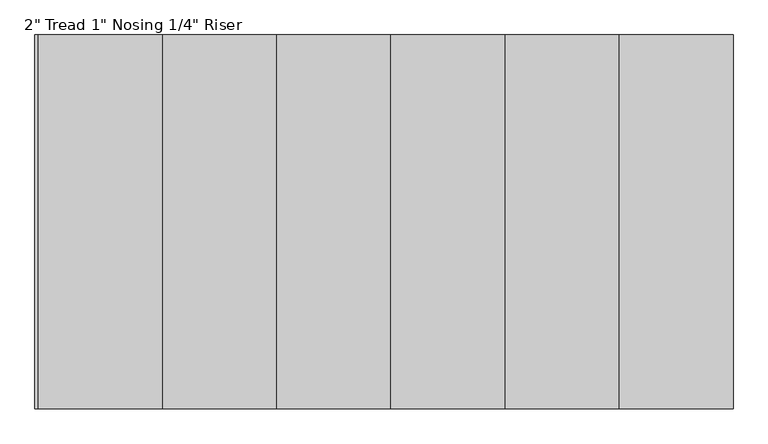
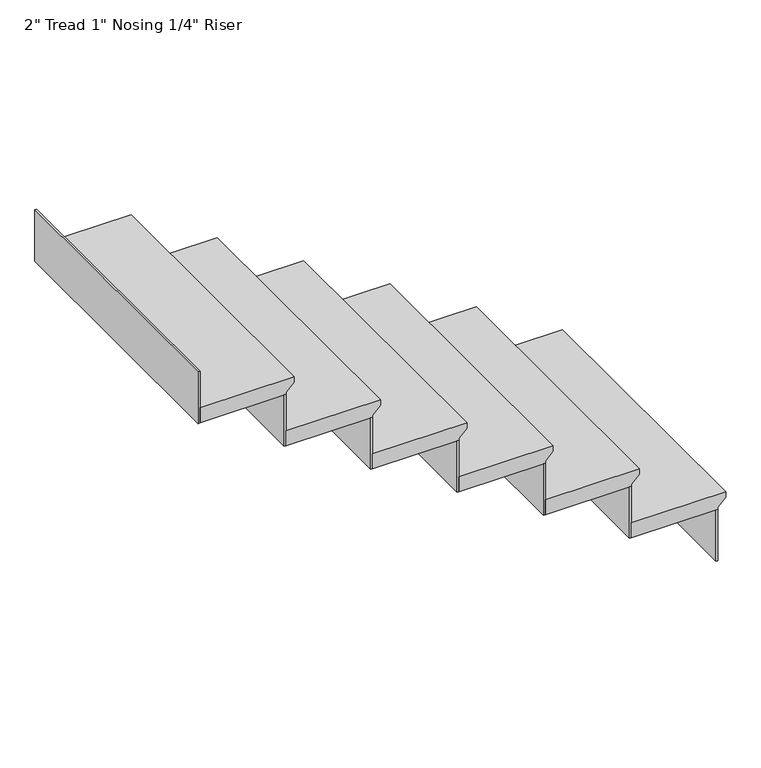
"""IFC4 building model written with IfcOpenShell, lengths in millimetres: stair flight geometry."""

from ifc_helpers import new_model, si_unit, frame, origin, place, context, project, spatial, polyline, outline, extrude, source, transform, mapped, element, save


def stair_flight_883e4480(model_context):
    return source(origin(), model_context, "Body", "SweptSolid", [
        extrude(outline(polyline([(2294.0210526, 8676.6463344), (2294.0210526, 8371.8463344), (2243.2210526, 8371.8463344), (2243.2210526, 8651.2463344), (2249.5710526, 8651.2463344), (2274.9710526, 8676.6463344), (2294.0210526, 8676.6463344)])), frame((0.0, -8089.9746824, 0.0), z_axis=(0.0, 1.0, 0.0), x_axis=(0.0, 0.0, 1.0)), (0.0, 0.0, 1.0), 914.4),
        extrude(outline(polyline([(8644.8963344, -7175.5746824), (8651.2463344, -7175.5746824), (8651.2463344, -8089.9746824), (8644.8963344, -8089.9746824), (8644.8963344, -7175.5746824)])), frame((0.0, 0.0, 2066.7578947), z_axis=(0.0, 0.0, 1.0), x_axis=(1.0, 0.0, 0.0)), (0.0, 0.0, 1.0), 176.4631579),
        extrude(outline(polyline([(8365.4963344, -7175.5746824), (8371.8463344, -7175.5746824), (8371.8463344, -8089.9746824), (8365.4963344, -8089.9746824), (8365.4963344, -7175.5746824)])), frame((0.0, 0.0, 2243.2210526), z_axis=(0.0, 0.0, 1.0), x_axis=(1.0, 0.0, 0.0)), (0.0, 0.0, 1.0), 176.4631579),
        extrude(outline(polyline([(2470.4842105, 8397.2463344), (2470.4842105, 8092.4463344), (2419.6842105, 8092.4463344), (2419.6842105, 8371.8463344), (2426.0342105, 8371.8463344), (2451.4342105, 8397.2463344), (2470.4842105, 8397.2463344)])), frame((0.0, -8089.9746824, 0.0), z_axis=(0.0, 1.0, 0.0), x_axis=(0.0, 0.0, 1.0)), (0.0, 0.0, 1.0), 914.4),
        extrude(outline(polyline([(8086.0963344, -7175.5746824), (8092.4463344, -7175.5746824), (8092.4463344, -8089.9746824), (8086.0963344, -8089.9746824), (8086.0963344, -7175.5746824)])), frame((0.0, 0.0, 2419.6842105), z_axis=(0.0, 0.0, 1.0), x_axis=(1.0, 0.0, 0.0)), (0.0, 0.0, 1.0), 176.4631579),
        extrude(outline(polyline([(2646.9473684, 8117.8463344), (2646.9473684, 7813.0463344), (2596.1473684, 7813.0463344), (2596.1473684, 8092.4463344), (2602.4973684, 8092.4463344), (2627.8973684, 8117.8463344), (2646.9473684, 8117.8463344)])), frame((0.0, -8089.9746824, 0.0), z_axis=(0.0, 1.0, 0.0), x_axis=(0.0, 0.0, 1.0)), (0.0, 0.0, 1.0), 914.4),
        extrude(outline(polyline([(7806.6963344, -7175.5746824), (7813.0463344, -7175.5746824), (7813.0463344, -8089.9746824), (7806.6963344, -8089.9746824), (7806.6963344, -7175.5746824)])), frame((0.0, 0.0, 2596.1473684), z_axis=(0.0, 0.0, 1.0), x_axis=(1.0, 0.0, 0.0)), (0.0, 0.0, 1.0), 176.4631579),
        extrude(outline(polyline([(2823.4105263, 7838.4463344), (2823.4105263, 7533.6463344), (2772.6105263, 7533.6463344), (2772.6105263, 7813.0463344), (2778.9605263, 7813.0463344), (2804.3605263, 7838.4463344), (2823.4105263, 7838.4463344)])), frame((0.0, -8089.9746824, 0.0), z_axis=(0.0, 1.0, 0.0), x_axis=(0.0, 0.0, 1.0)), (0.0, 0.0, 1.0), 914.4),
        extrude(outline(polyline([(7527.2963344, -7175.5746824), (7533.6463344, -7175.5746824), (7533.6463344, -8089.9746824), (7527.2963344, -8089.9746824), (7527.2963344, -7175.5746824)])), frame((0.0, 0.0, 2772.6105263), z_axis=(0.0, 0.0, 1.0), x_axis=(1.0, 0.0, 0.0)), (0.0, 0.0, 1.0), 176.4631579),
        extrude(outline(polyline([(2999.8736842, 7559.0463344), (2999.8736842, 7254.2463344), (2949.0736842, 7254.2463344), (2949.0736842, 7533.6463344), (2955.4236842, 7533.6463344), (2980.8236842, 7559.0463344), (2999.8736842, 7559.0463344)])), frame((0.0, -8089.9746824, 0.0), z_axis=(0.0, 1.0, 0.0), x_axis=(0.0, 0.0, 1.0)), (0.0, 0.0, 1.0), 914.4),
        extrude(outline(polyline([(7247.8963344, -7175.5746824), (7254.2463344, -7175.5746824), (7254.2463344, -8089.9746824), (7247.8963344, -8089.9746824), (7247.8963344, -7175.5746824)])), frame((0.0, 0.0, 2949.0736842), z_axis=(0.0, 0.0, 1.0), x_axis=(1.0, 0.0, 0.0)), (0.0, 0.0, 1.0), 176.4631579),
        extrude(outline(polyline([(6968.4963344, -7175.5746824), (6974.8463344, -7175.5746824), (6974.8463344, -8089.9746824), (6968.4963344, -8089.9746824), (6968.4963344, -7175.5746824)])), frame((0.0, 0.0, 3125.5368421), z_axis=(0.0, 0.0, 1.0), x_axis=(1.0, 0.0, 0.0)), (0.0, 0.0, 1.0), 176.4631579),
        extrude(outline(polyline([(3176.3368421, 7279.6463344), (3176.3368421, 6974.8463344), (3125.5368421, 6974.8463344), (3125.5368421, 7254.2463344), (3131.8868421, 7254.2463344), (3157.2868421, 7279.6463344), (3176.3368421, 7279.6463344)])), frame((0.0, -8089.9746824, 0.0), z_axis=(0.0, 1.0, 0.0), x_axis=(0.0, 0.0, 1.0)), (0.0, 0.0, 1.0), 914.4),
    ])


if __name__ == "__main__":
    model = new_model("IFC4")
    model_context = context("Model", 3, world=origin())
    ifc_project = project(units=[si_unit("LENGTHUNIT", "METRE", prefix="MILLI")], contexts=[model_context])
    site = spatial("IfcSite", under=ifc_project)
    building = spatial("IfcBuilding", under=site)
    placement = place(None, origin())
    stair_flight_shape = stair_flight_883e4480(model_context)
    element("IfcStairFlight", 1, ObjectType="2\" Tread 1\" Nosing 1/4\" Riser", at=placement, inside=building, context=model_context, shape_type="MappedRepresentation", body=[
        mapped(stair_flight_shape, transform((0.0, 0.0, 0.0), x_axis=(1.0, 0.0, 0.0), y_axis=(0.0, 1.0, 0.0), z_axis=(0.0, 0.0, 1.0))),
    ])
    save(model, "model.ifc")

# Revit data of these elements
# Element 1 (IfcStairFlight, "2\" Tread 1\" Nosing 1/4\" Riser")
#   Materials on its faces: "MARBLE STAIRS 6\""
# Materials
#   "MARBLE STAIRS 6\"": class "Generic", colour RGB 120 120 120, transparency 0, Cost = 0
